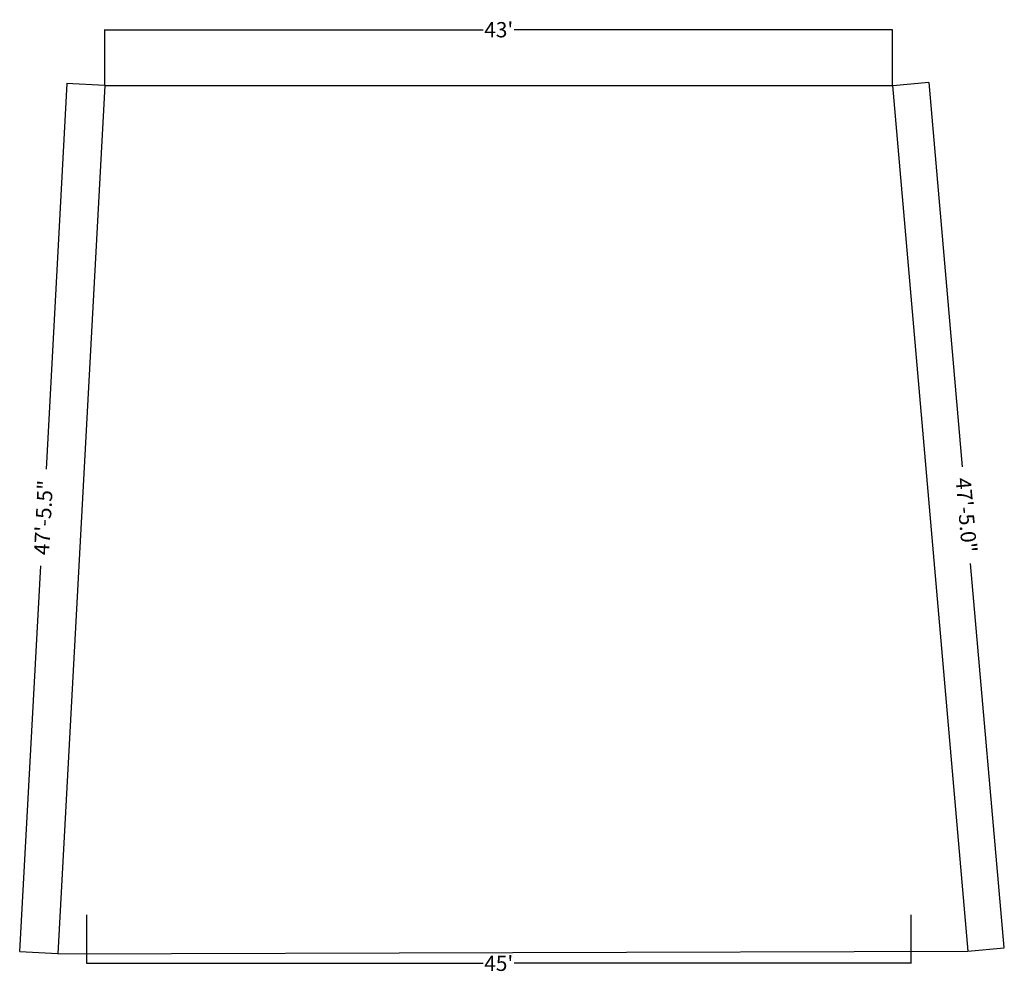
# Model space of a CAD drawing. Units: inches. Extents: x -269 to 4574, y -694 to 313.
# Tile 19 of 19: x 3929 to 4574, y -579 to 46. Entities that reach past the tile are written whole.
import ezdxf

# ---------------------------------------------------------------- set-up
doc = ezdxf.new("R2010")
doc.units = ezdxf.units.IN
doc.header["$MEASUREMENT"] = 0
doc.layers.add('C-PROP', color=7, linetype='Continuous', lineweight=25)
doc.layers.add('DIMENSION', color=5, linetype='Continuous', lineweight=18)
doc.dimstyles.get("Standard").update_dxf_attribs({"dimtxt": 10, "dimasz": 0.18, "dimexe": 0.18, "dimexo": 0.0625, "dimgap": 0.09, "dimtad": 0, "dimdec": 1, "dimzin": 0, "dimdsep": 46, "dimlunit": 3, "dimtxsty": 'Standard', "dimcen": 0.09, "dimclrt": 7, "dimadec": 0, "dimazin": 0, "dimtfac": 1, "dimtdec": 1, "dimtofl": 0, "dimtmove": 0, "dimatfit": 3, "dimfxl": 1, "dimtolj": 1, "dimtzin": 0, "dimarcsym": 0})

# ---------------------------------------------------------------- blocks, each defined once
blk = doc.blocks.new('*D28')
at = {"layer": 'Defpoints', "color": 0, "lineweight": 0, "transparency": 16777216}
for p in [(3984.55, 2.57), (3928.94, -564.75), (3953.8, -566.1)]:
    blk.add_point(p, dxfattribs=at)
at = {"layer": 'DIMENSION', "color": 0, "lineweight": -2, "transparency": 16777216}
for p, q in [((3959.67, 3.74), (3946.02, -248.71)), ((3984.48, 2.58), (3959.5, 3.93)), ((3928.94, -564.57), (3942.59, -312.13)), ((3953.74, -566.09), (3928.76, -564.74))]:
    blk.add_line(p, q, dxfattribs=at)
at = {"layer": 'DIMENSION', "color": 0, "lineweight": 0, "transparency": 16777216}
for points in [[(3959.64, 3.74), (3959.7, 3.74), (3959.68, 3.92)], [(3928.92, -564.57), (3928.97, -564.57), (3928.94, -564.75)]]:
    blk.add_solid(points, dxfattribs=at)
at = {"layer": 'DIMENSION', "color": 0, "transparency": 16777216, "insert": (3944.31, -280.42), "char_height": 10, "attachment_point": 5, "rotation": 86.90535}
blk.add_mtext('\\A1;47\'-5.5"', dxfattribs=at)
blk = doc.blocks.new('*D29')
at = {"layer": 'Defpoints', "color": 0, "lineweight": 0, "transparency": 16777216}
for p in [(4500.55, 2.57), (4549.88, -564.28), (4573.55, -562.22)]:
    blk.add_point(p, dxfattribs=at)
at = {"layer": 'DIMENSION', "color": 0, "lineweight": -2, "transparency": 16777216}
for p, q in [((4500.61, 2.58), (4524.39, 4.65)), ((4524.23, 4.45), (4546.13, -247.16)), ((4573.53, -562.04), (4551.63, -310.43)), ((4549.94, -564.28), (4573.73, -562.21))]:
    blk.add_line(p, q, dxfattribs=at)
at = {"layer": 'DIMENSION', "color": 0, "lineweight": 0, "transparency": 16777216}
for points in [[(4524.26, 4.46), (4524.2, 4.45), (4524.21, 4.63)], [(4573.56, -562.04), (4573.5, -562.05), (4573.55, -562.22)]]:
    blk.add_solid(points, dxfattribs=at)
at = {"layer": 'DIMENSION', "color": 0, "transparency": 16777216, "insert": (4548.88, -278.8), "char_height": 10, "attachment_point": 5, "rotation": 274.97381}
blk.add_mtext('\\A1;47\'-5.0"', dxfattribs=at)
blk = doc.blocks.new('*D30')
at = {"layer": 'Defpoints', "color": 0, "lineweight": 0, "transparency": 16777216}
for p in [(3972.55, -540.52), (4512.55, -540.52), (4512.55, -572.31)]:
    blk.add_point(p, dxfattribs=at)
at = {"layer": 'DIMENSION', "color": 0, "lineweight": -2, "transparency": 16777216}
for p, q in [((3972.55, -540.59), (3972.55, -572.49)), ((4512.55, -540.59), (4512.55, -572.49)), ((3972.73, -572.31), (4232.46, -572.31)), ((4512.37, -572.31), (4252.64, -572.31))]:
    blk.add_line(p, q, dxfattribs=at)
at = {"layer": 'DIMENSION', "color": 0, "lineweight": 0, "transparency": 16777216}
for points in [[(3972.73, -572.28), (3972.73, -572.34), (3972.55, -572.31)], [(4512.37, -572.28), (4512.37, -572.34), (4512.55, -572.31)]]:
    blk.add_solid(points, dxfattribs=at)
at = {"layer": 'DIMENSION', "color": 0, "transparency": 16777216, "insert": (4242.55, -572.31), "char_height": 10, "attachment_point": 5}
blk.add_mtext("\\A1;45'", dxfattribs=at)
blk = doc.blocks.new('*D31')
at = {"layer": 'Defpoints', "color": 0, "lineweight": 0, "transparency": 16777216}
for p in [(4500.55, 39.06), (3984.55, 2.57), (4500.55, 2.57)]:
    blk.add_point(p, dxfattribs=at)
at = {"layer": 'DIMENSION', "color": 0, "lineweight": -2, "transparency": 16777216}
for p, q in [((3984.55, 2.64), (3984.55, 39.24)), ((3984.73, 39.06), (4232.46, 39.06)), ((4500.37, 39.06), (4252.64, 39.06)), ((4500.55, 2.64), (4500.55, 39.24))]:
    blk.add_line(p, q, dxfattribs=at)
at = {"layer": 'DIMENSION', "color": 0, "lineweight": 0, "transparency": 16777216}
for points in [[(3984.73, 39.09), (3984.73, 39.03), (3984.55, 39.06)], [(4500.37, 39.09), (4500.37, 39.03), (4500.55, 39.06)]]:
    blk.add_solid(points, dxfattribs=at)
at = {"layer": 'DIMENSION', "color": 0, "transparency": 16777216, "insert": (4242.55, 39.06), "char_height": 10, "attachment_point": 5}
blk.add_mtext("\\A1;43'", dxfattribs=at)

msp = doc.modelspace()

# ---------------------------------------------------------------- linework, layer by layer
at = {"layer": 'C-PROP'}
for p, q in [((3984.55, 2.57), (3953.8, -566.1)), ((3984.55, 2.57), (4500.55, 2.57)), ((4500.55, 2.57), (4549.88, -564.28)), ((3953.8, -566.1), (4549.88, -564.28))]:
    msp.add_line(p, q, dxfattribs=at)

# ---------------------------------------------------------------- dimensions: what is measured, and where the dimension line sits
at = {"layer": 'DIMENSION'}
for base, p1, p2, picture, middle in [((4500.55, 39.06), (3984.55, 2.57), (4500.55, 2.57), '*D31', (4242.55, 39.06)), ((4512.55, -572.31), (3972.55, -540.52), (4512.55, -540.52), '*D30', (4242.55, -572.31))]:
    dim = msp.add_linear_dim(base=base, p1=p1, p2=p2, dimstyle='Standard', override={"dimclrd": 0, "dimclre": 0, "dimclrt": 0}, dxfattribs=at)
    dim.commit()
    dim.dimension.update_dxf_attribs({"geometry": picture, "text_midpoint": middle})
for p1, p2, distance, picture, middle in [((3984.55, 2.57), (3953.8, -566.1), -24.9, '*D28', (3944.31, -280.42)), ((4500.55, 2.57), (4549.88, -564.28), 23.76, '*D29', (4548.88, -278.8))]:
    dim = msp.add_aligned_dim(p1=p1, p2=p2, distance=distance, dimstyle='Standard', override={"dimclrd": 0, "dimclre": 0, "dimclrt": 0}, dxfattribs=at)
    dim.commit()
    dim.dimension.update_dxf_attribs({"geometry": picture, "text_midpoint": middle})

doc.saveas('drawing.dxf')
